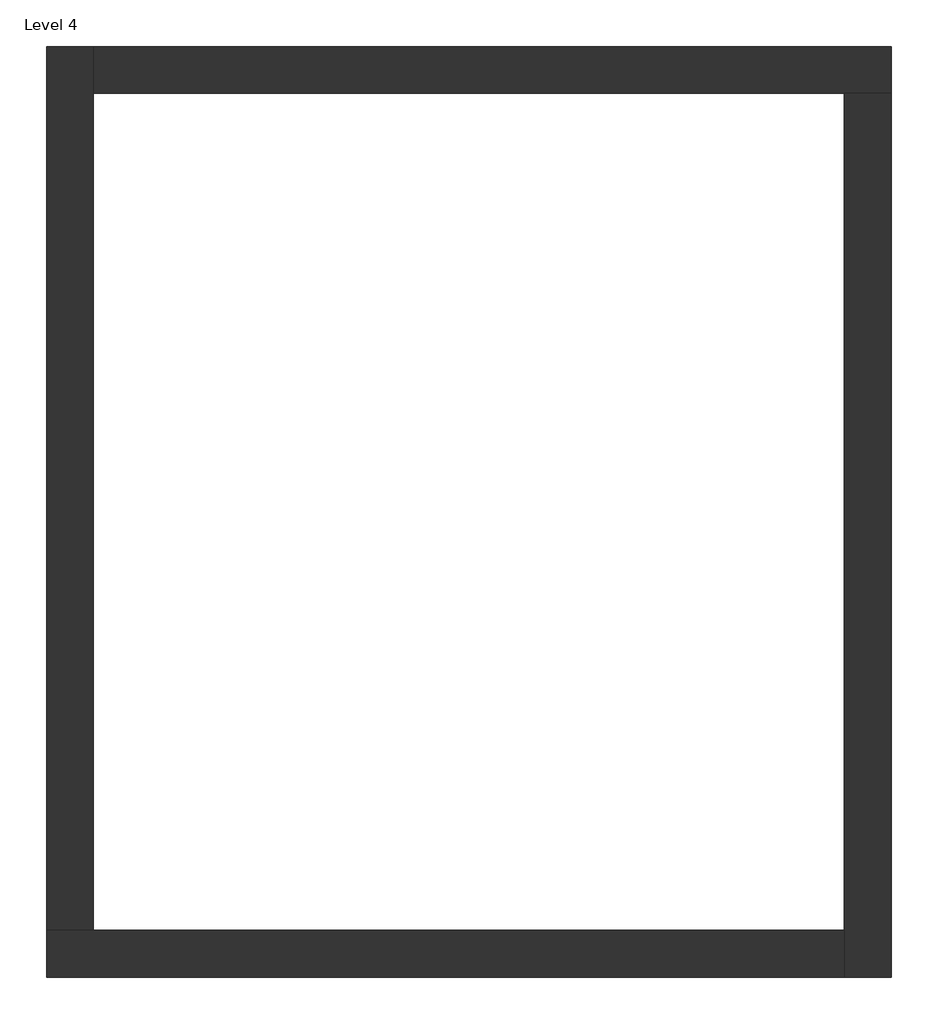
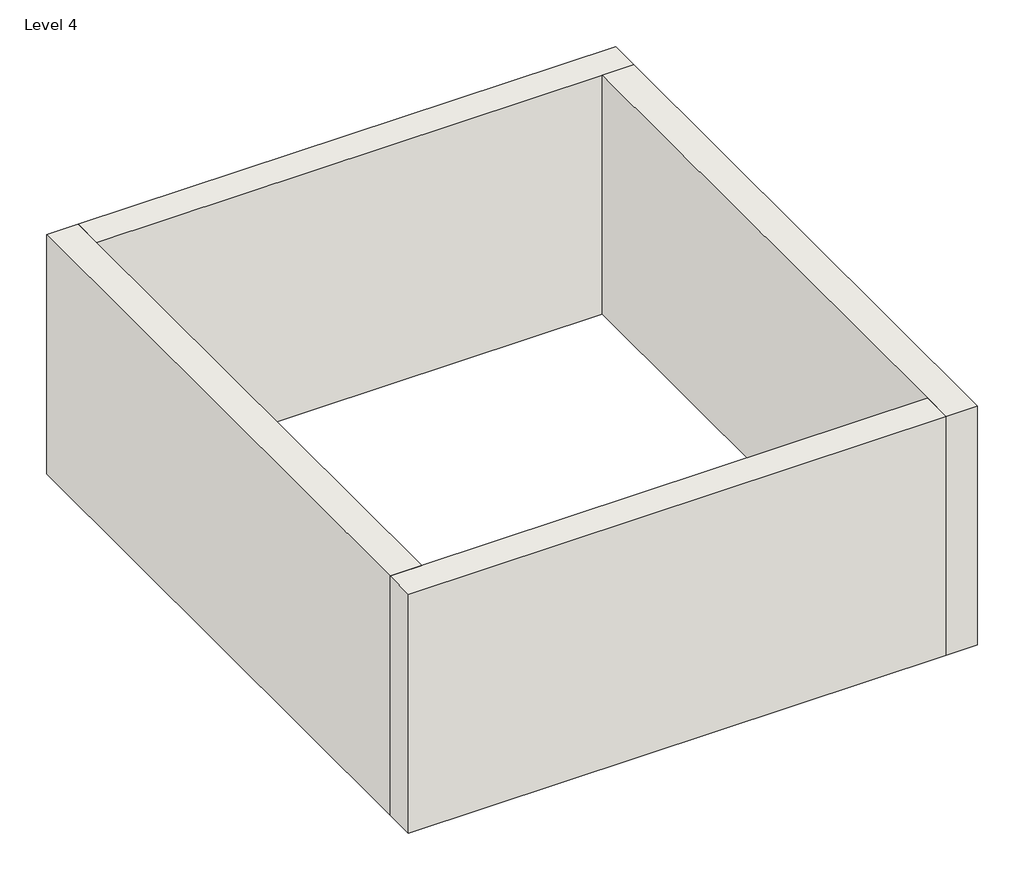
# One storey: 4 walls.
"""IFC4 building model written with IfcOpenShell, lengths in millimetres."""

from ifc_helpers import new_model, si_unit, origin, place, context, project, spatial, faceted_brep, element, save

model = new_model("IFC4")

# Units and contexts
model_context = context("Model", 3, world=origin())
ifc_project = project(units=[si_unit("LENGTHUNIT", "METRE", prefix="MILLI")], contexts=[model_context])

# Site, building, storey
site = spatial("IfcSite", under=ifc_project)
building = spatial("IfcBuilding", under=site)
storey = spatial("IfcBuildingStorey", under=building, Name="Level 4", Elevation=3810.0)

# Walls
placement = place(None, origin())
element("IfcWall", 1, ObjectType="9\" wall", at=placement, inside=storey, context=model_context, shape_type="Brep", body=[
    faceted_brep([(4952.0424957, 9460.5408272, 3810.0), (1065.8424957, 9460.5408272, 3810.0), (1065.8424957, 9460.5408272, 5638.8), (4952.0424957, 9460.5408272, 5638.8), (4952.0424957, 9231.9408272, 3810.0), (4952.0424957, 9231.9408272, 5638.8), (4723.4424957, 9231.9408272, 5638.8), (1065.8424957, 9231.9408272, 5638.8), (1065.8424957, 9231.9408272, 3810.0), (4723.4424957, 9231.9408272, 3810.0)], [[[0, 1, 2, 3]], [[4, 5, 6, 7, 8, 9]], [[1, 0, 4, 9, 8]], [[3, 2, 7, 6, 5]], [[0, 3, 5, 4]], [[2, 1, 8, 7]]]),
])
element("IfcWall", 2, ObjectType="9\" wall", at=placement, inside=storey, context=model_context, shape_type="Brep", body=[
    faceted_brep([(4952.0424957, 4926.6408272, 3810.0), (4952.0424957, 9231.9408272, 3810.0), (4952.0424957, 9231.9408272, 5638.8), (4952.0424957, 4926.6408272, 5638.8), (4723.4424957, 4926.6408272, 3810.0), (4723.4424957, 4926.6408272, 5638.8), (4723.4424957, 5155.2408272, 5638.8), (4723.4424957, 9231.9408272, 5638.8), (4723.4424957, 9231.9408272, 3810.0), (4723.4424957, 5155.2408272, 3810.0)], [[[0, 1, 2, 3]], [[4, 5, 6, 7, 8, 9]], [[1, 0, 4, 9, 8]], [[3, 2, 7, 6, 5]], [[0, 3, 5, 4]], [[2, 1, 8, 7]]]),
])
element("IfcWall", 3, ObjectType="9\" wall", at=placement, inside=storey, context=model_context, shape_type="Brep", body=[
    faceted_brep([(837.2424957, 4926.6408272, 3810.0), (4723.4424957, 4926.6408272, 3810.0), (4723.4424957, 4926.6408272, 5638.8), (837.2424957, 4926.6408272, 5638.8), (837.2424957, 5155.2408272, 3810.0), (837.2424957, 5155.2408272, 5638.8), (1065.8424957, 5155.2408272, 5638.8), (4723.4424957, 5155.2408272, 5638.8), (4723.4424957, 5155.2408272, 3810.0), (1065.8424957, 5155.2408272, 3810.0)], [[[0, 1, 2, 3]], [[4, 5, 6, 7, 8, 9]], [[1, 0, 4, 9, 8]], [[3, 2, 7, 6, 5]], [[0, 3, 5, 4]], [[2, 1, 8, 7]]]),
])
element("IfcWall", 4, ObjectType="9\" wall", at=placement, inside=storey, context=model_context, shape_type="Brep", body=[
    faceted_brep([(837.2424957, 9460.5408272, 3810.0), (837.2424957, 5155.2408272, 3810.0), (837.2424957, 5155.2408272, 5638.8), (837.2424957, 9460.5408272, 5638.8), (1065.8424957, 9460.5408272, 3810.0), (1065.8424957, 9460.5408272, 5638.8), (1065.8424957, 9231.9408272, 5638.8), (1065.8424957, 5155.2408272, 5638.8), (1065.8424957, 5155.2408272, 3810.0), (1065.8424957, 9231.9408272, 3810.0)], [[[0, 1, 2, 3]], [[4, 5, 6, 7, 8, 9]], [[1, 0, 4, 9, 8]], [[3, 2, 7, 6, 5]], [[0, 3, 5, 4]], [[2, 1, 8, 7]]]),
])

save(model, "model.ifc")

# Revit data of these elements
# Type "9\" wall"
#   Assembly Code = "B2010"
#   Layers, outside or top first: 0' - 9" "wall" (function 1)
# Elements 1, 2, 3, 4 (IfcWall, "9\" wall")
#   Top Offset = 0' - 0"
#   Base Offset = 0' - 0"
#   Unconnected Height = 6' - 0"
#   wall height = 6' - 0"
#   Phase Created = New Construction
#   Base Constraint = Level 4
#   Materials on its faces: "wall"
# Materials
#   "wall": class "Generic", colour RGB 120 120 120, transparency 0, Cost = 0
